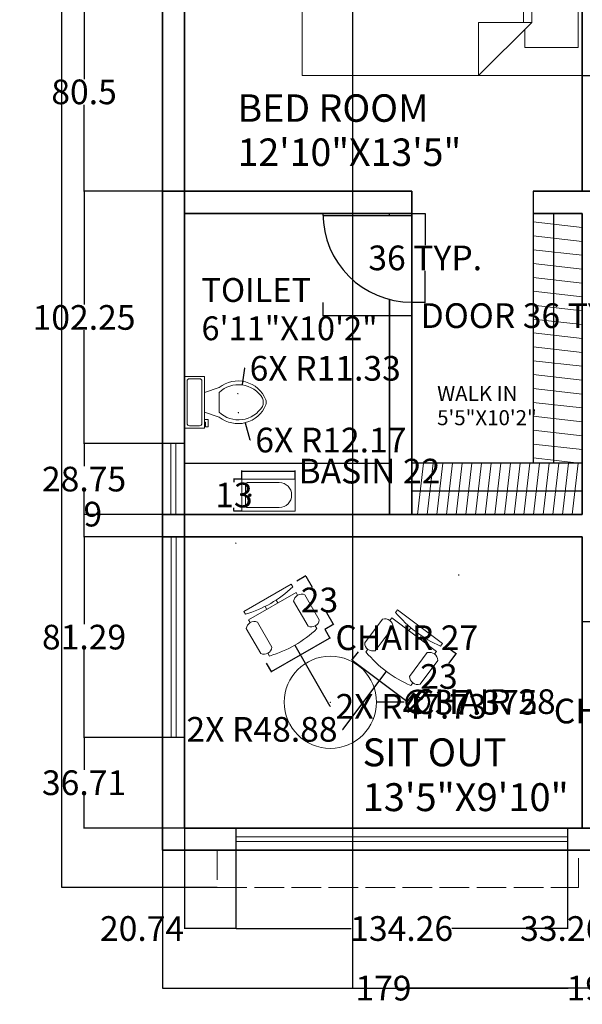
# Model space of a CAD drawing. Units: inches. Extents: x 135 to 880, y 60 to 879.
# Tile 1 of 5: x 135 to 363, y 60 to 459. Entities that reach past the tile are written whole.
import ezdxf

# ---------------------------------------------------------------- set-up
doc = ezdxf.new("R2010")
doc.units = ezdxf.units.IN
doc.header["$MEASUREMENT"] = 0
doc.linetypes.add('ACAD_ISO02W100', pattern=[15, 12, -3])
for name, color, linetype, lineweight in [('A-ANNO-DIMS', 2, 'Continuous', 18), ('A-AREA-IDEN', 7, 'Continuous', 18), ('A-DOOR', 3, 'Continuous', 25), ('A-FLOR-CASE', 32, 'Continuous', 25), ('A-FLOR-CASE-PATT', 252, 'Continuous', 13), ('A-FLOR-FIXT', 9, 'Continuous', 20), ('A-FURN', 8, 'Continuous', 18), ('A-GLAZ', 4, 'Continuous', 18), ('A-ROOF-OVHD', 8, 'ACAD_ISO02W100', 18), ('A-WALL', 7, 'Continuous', 35)]:
    doc.layers.add(name, color=color, linetype=linetype, lineweight=lineweight)
doc.styles.get("Standard").update_dxf_attribs({"font": 'arial.ttf'})
doc.dimstyles.get("Standard").update_dxf_attribs({"dimtxt": 10, "dimasz": 0.18, "dimexe": 0.18, "dimexo": 0.0625, "dimgap": 0.09, "dimtad": 0, "dimtih": 1, "dimtoh": 1, "dimdec": 0, "dimzin": 0, "dimdsep": 46, "dimlunit": 3, "dimtxsty": 'Standard', "dimcen": 0.09, "dimadec": 0, "dimazin": 0, "dimtfac": 1, "dimtdec": 0, "dimtofl": 0, "dimtmove": 0, "dimatfit": 3, "dimfxl": 1, "dimtolj": 1, "dimtzin": 0, "dimarcsym": 0})

# ---------------------------------------------------------------- blocks, each defined once
blk = doc.blocks.new('Chair - Desk')
for p, q in [((-8.5, 0), (-8.5, -1)), ((-8.5, 0), (8.5, 0)), ((8.5, 0), (8.5, -1)), ((-2, -3), (-2, -1.9355)), ((2, -1.9576), (2, -3)), ((-10.5, -5), (-10.5, -14)), ((-8.5, -3), (-8.5, -4)), ((-8.5, -3), (8.5, -3)), ((-6.5, -14), (-6.5, -5)), ((6.5, -5), (6.5, -14)), ((8.5, -3), (8.5, -4)), ((10.5, -14), (10.5, -5)), ((-8.5, -15), (-8.5, -16)), ((8.5, -15), (8.5, -16))]:
    blk.add_line(p, q)
for centre, radius, start, end in [((0, 34.625), 36.625, 256.5803, 283.4197), ((-8.5, -6.5), 2.5, 36.8699, 143.1301), ((8.5, -6.5), 2.5, 36.8699, 143.1301), ((-8.5, -12.5), 2.5, 216.8699, 323.1301), ((8.5, -12.5), 2.5, 216.8699, 323.1301), ((0, 19.625), 36.625, 256.5803, 283.4197)]:
    blk.add_arc(centre, radius, start, end)
blk = doc.blocks.new('Bed - Queen')
for p, q in [((0, -80.00003), (0, 0)), ((0, 0), (59.99999, 0)), ((59.99999, 0), (59.99999, -80.00003)), ((7.99999, -1.2), (28.79998, -1.2)), ((7.99999, -14.4), (7.99999, -1.2)), ((28.79998, -1.2), (28.79998, -14.4)), ((31.19999, -1.2), (51.99999, -1.2)), ((31.19999, -14.4), (31.19999, -1.2)), ((51.99999, -1.2), (51.99999, -16.4)), ((0, -14.4), (44.8, -14.4)), ((44.8, -16.8), (0, -16.8)), ((59.99999, -29.6), (44.8, -14.4)), ((44.8, -14.4), (44.8, -29.6)), ((51.99999, -16.4), (46.79936, -16.4)), ((44.8, -29.6), (59.99999, -29.6)), ((59.99999, -80.00003), (0, -80.00003))]:
    blk.add_line(p, q)
blk = doc.blocks.new('Toilet - top')
for p, q in [((9.5, -6), (9.5, -2)), ((-10, -8.5), (-8, -8.5)), ((-10, -9.5), (-10, -8.5)), ((-7, -9.5), (-10, -9.5)), ((-8, -8.5), (-8, -8)), ((-7, -8), (-7, -9.5)), ((-4, -8), (-6, -14)), ((4, -8), (6, -14)), ((4, -14), (-4, -14))]:
    blk.add_line(p, q)
blk.add_lwpolyline([(10.5, -8), (10.5, 0), (-10.5, 0), (-10.5, -8)], close=True)
for points in [[(-9.5, -2), (-9.5, -6)], [(8.5, -1), (-8.5, -1)], [(-8.5, -7), (8.5, -7)]]:
    blk.add_lwpolyline(points)
for centre, radius, start, end in [((-8.62, -1.88), 0.884, 81.8699, 188.1301), ((8.62, -1.88), 0.884, 351.8699, 98.1301), ((-8.62, -6.12), 0.884, 171.8699, 278.1301), ((8.62, -6.12), 0.884, 261.8699, 8.1301), ((3.52, -21.58), 12.17, 141.4691, 247.9714), ((4.2, -21.82), 11.33, 136.3677, 238.9468), ((-3.52, -21.58), 12.17, 292.0284, 38.5307), ((-4.2, -21.82), 11.33, 301.053, 43.6321), ((0, -27.88), 4, 245.7318, 294.2682), ((0, -29), 4, 254.8605, 285.1395)]:
    blk.add_arc(centre, radius, start, end)
blk = doc.blocks.new('Bath Tub - 26 x 60 in.')
for p, q in [((8, -18), (10, -18)), ((9, -17), (9, -19))]:
    blk.add_line(p, q)
blk.add_lwpolyline([(0, -36), (0, 0), (60, 0), (60, -36)], close=True)
for points in [[(4, -30), (4, -6)], [(6, -4), (42, -4)], [(42, -32), (6, -32)]]:
    blk.add_lwpolyline(points)
for radius in [1.5, 1]:
    blk.add_circle((9, -18), radius)
for centre, radius, start, end in [((5.75, -5.75), 1.77, 81.8699, 188.1301), ((42, -18), 14, 270, 90), ((5.75, -30.25), 1.77, 171.8699, 278.1301)]:
    blk.add_arc(centre, radius, start, end)
blk = doc.blocks.new('DOOR-SWING-36IN')
for p, q in [((36, 36), (0, 36)), ((36, 35), (0, 35))]:
    blk.add_line(p, q)
blk.add_arc((36, 36), 36, 180, 270)
blk = doc.blocks.new('*D8')
at = {"layer": 'A-ANNO-DIMS', "color": 0, "lineweight": -2, "transparency": 16777216}
for p, q in [((258.71, 212.22), (260.83, 208.57)), ((237.19, 195.13), (260.58, 208.63)), ((260.74, 208.72), (260.89, 208.81)), ((260.89, 208.81), (261.07, 208.81)), ((235.02, 198.54), (237.13, 194.89))]:
    blk.add_line(p, q, dxfattribs=at)
at = {"layer": 'A-ANNO-DIMS', "color": 0, "transparency": 16777216}
for points in [[(260.56, 208.66), (260.59, 208.61), (260.74, 208.72)], [(237.18, 195.16), (237.21, 195.11), (237.04, 195.04)]]:
    blk.add_solid(points, dxfattribs=at)
at = {"layer": 'Defpoints', "color": 0, "transparency": 16777216}
for p in [(258.68, 212.28), (260.74, 208.72), (234.98, 198.6)]:
    blk.add_point(p, dxfattribs=at)
at = {"layer": 'A-ANNO-DIMS', "color": 0, "transparency": 16777216, "insert": (291.94, 208.81), "char_height": 10, "attachment_point": 5}
blk.add_mtext('\\A1;CHAIR 27', dxfattribs=at)
blk = doc.blocks.new('*D9')
at = {"layer": 'A-ANNO-DIMS', "color": 0, "lineweight": -2, "transparency": 16777216}
for p, q in [((247.44, 231.87), (251.1, 233.98)), ((251.03, 233.74), (253.59, 229.31)), ((262.15, 214.49), (259.59, 218.91)), ((258.74, 212.31), (262.39, 214.42))]:
    blk.add_line(p, q, dxfattribs=at)
at = {"layer": 'A-ANNO-DIMS', "color": 0, "transparency": 16777216}
for points in [[(251.06, 233.75), (251.01, 233.72), (250.94, 233.89)], [(262.17, 214.5), (262.12, 214.47), (262.24, 214.33)]]:
    blk.add_solid(points, dxfattribs=at)
at = {"layer": 'Defpoints', "color": 0, "transparency": 16777216}
for p in [(247.39, 231.84), (250.94, 233.89), (258.68, 212.28)]:
    blk.add_point(p, dxfattribs=at)
at = {"layer": 'A-ANNO-DIMS', "color": 0, "transparency": 16777216, "insert": (256.59, 224.11), "char_height": 10, "attachment_point": 5}
blk.add_mtext('\\A1;23', dxfattribs=at)
blk = doc.blocks.new('*D10')
at = {"layer": 'A-ANNO-DIMS', "color": 0, "lineweight": -2, "transparency": 16777216}
for p, q in [((272.18, 203.16), (269.58, 199.7)), ((269.83, 199.74), (291.97, 183.14)), ((294.59, 186.34), (292, 182.88)), ((292.11, 183.03), (292.25, 182.92)), ((292.25, 182.92), (292.43, 182.92))]:
    blk.add_line(p, q, dxfattribs=at)
at = {"layer": 'A-ANNO-DIMS', "color": 0, "transparency": 16777216}
for points in [[(269.85, 199.76), (269.82, 199.71), (269.69, 199.84)], [(291.98, 183.16), (291.95, 183.11), (292.11, 183.03)]]:
    blk.add_solid(points, dxfattribs=at)
at = {"layer": 'Defpoints', "color": 0, "transparency": 16777216}
for p in [(272.21, 203.21), (294.63, 186.39), (292.11, 183.03)]:
    blk.add_point(p, dxfattribs=at)
at = {"layer": 'A-ANNO-DIMS', "color": 0, "transparency": 16777216, "insert": (323.31, 182.92), "char_height": 10, "attachment_point": 5}
blk.add_mtext('\\A1;CHAIR 28', dxfattribs=at)
blk = doc.blocks.new('*D11')
at = {"layer": 'A-ANNO-DIMS', "color": 0, "lineweight": -2, "transparency": 16777216}
for p, q in [((308.56, 204.86), (312.02, 202.27)), ((311.77, 202.23), (308.83, 198.32)), ((298.1, 184.01), (301.03, 187.92)), ((294.68, 186.35), (298.14, 183.76))]:
    blk.add_line(p, q, dxfattribs=at)
at = {"layer": 'A-ANNO-DIMS', "color": 0, "transparency": 16777216}
for points in [[(311.74, 202.25), (311.79, 202.21), (311.87, 202.37)], [(298.08, 184.03), (298.13, 184), (297.99, 183.87)]]:
    blk.add_solid(points, dxfattribs=at)
at = {"layer": 'Defpoints', "color": 0, "transparency": 16777216}
for p in [(308.51, 204.9), (311.87, 202.37), (294.63, 186.39)]:
    blk.add_point(p, dxfattribs=at)
at = {"layer": 'A-ANNO-DIMS', "color": 0, "transparency": 16777216, "insert": (304.93, 193.12), "char_height": 10, "attachment_point": 5}
blk.add_mtext('\\A1;23', dxfattribs=at)
blk = doc.blocks.new('*D14')
at = {"layer": 'A-ANNO-DIMS', "color": 0, "lineweight": -2, "transparency": 16777216}
for p, q in [((454.9, 202.13), (411.72, 179.27)), ((458.48, 195.75), (454.97, 202.38)), ((411.4, 179.11), (411.22, 179.11)), ((411.56, 179.19), (411.4, 179.11)), ((414.99, 172.72), (411.48, 179.35))]:
    blk.add_line(p, q, dxfattribs=at)
at = {"layer": 'A-ANNO-DIMS', "color": 0, "transparency": 16777216}
for points in [[(454.88, 202.16), (454.91, 202.11), (455.05, 202.22)], [(411.71, 179.3), (411.73, 179.25), (411.56, 179.19)]]:
    blk.add_solid(points, dxfattribs=at)
at = {"layer": 'Defpoints', "color": 0, "transparency": 16777216}
for p in [(458.51, 195.69), (411.56, 179.19), (415.01, 172.67)]:
    blk.add_point(p, dxfattribs=at)
at = {"layer": 'A-ANNO-DIMS', "color": 0, "transparency": 16777216, "insert": (380.34, 179.11), "char_height": 10, "attachment_point": 5}
blk.add_mtext('\\A1;CHAIR 49', dxfattribs=at)
blk = doc.blocks.new('*D18')
at = {"layer": 'A-ANNO-DIMS', "color": 0, "lineweight": -2, "transparency": 16777216}
for p, q in [((225.19, 273.15), (225.19, 276.5)), ((225.37, 276.32), (246.58, 276.32)), ((246.76, 273.15), (246.76, 276.5)), ((246.76, 276.32), (246.94, 276.32))]:
    blk.add_line(p, q, dxfattribs=at)
at = {"layer": 'A-ANNO-DIMS', "color": 0, "transparency": 16777216}
for points in [[(225.37, 276.35), (225.37, 276.29), (225.19, 276.32)], [(246.58, 276.35), (246.58, 276.29), (246.76, 276.32)]]:
    blk.add_solid(points, dxfattribs=at)
at = {"layer": 'Defpoints', "color": 0, "transparency": 16777216}
for p in [(246.76, 276.32), (225.19, 273.08), (246.76, 273.08)]:
    blk.add_point(p, dxfattribs=at)
at = {"layer": 'A-ANNO-DIMS', "color": 0, "transparency": 16777216, "insert": (276.82, 276.32), "char_height": 10, "attachment_point": 5}
blk.add_mtext('\\A1;BASIN 22', dxfattribs=at)
blk = doc.blocks.new('*D19')
at = {"layer": 'A-ANNO-DIMS', "color": 0, "lineweight": -2, "transparency": 16777216}
for p, q in [((225.13, 273.08), (221.78, 273.08)), ((221.96, 272.9), (221.96, 271.81)), ((225.13, 260.15), (221.78, 260.15)), ((221.96, 260.33), (221.96, 261.42))]:
    blk.add_line(p, q, dxfattribs=at)
at = {"layer": 'A-ANNO-DIMS', "color": 0, "transparency": 16777216}
for points in [[(221.93, 272.9), (221.99, 272.9), (221.96, 273.08)], [(221.93, 260.33), (221.99, 260.33), (221.96, 260.15)]]:
    blk.add_solid(points, dxfattribs=at)
at = {"layer": 'Defpoints', "color": 0, "transparency": 16777216}
for p in [(221.96, 273.08), (225.19, 273.08), (225.19, 260.15)]:
    blk.add_point(p, dxfattribs=at)
at = {"layer": 'A-ANNO-DIMS', "color": 0, "transparency": 16777216, "insert": (221.96, 266.62), "char_height": 10, "attachment_point": 5}
blk.add_mtext('\\A1;13', dxfattribs=at)
blk = doc.blocks.new('*D25')
at = {"layer": 'A-ANNO-DIMS', "color": 0, "lineweight": -2, "transparency": 16777216}
for p, q in [((363.04, 521.66), (380.17, 521.66)), ((379.99, 521.48), (379.99, 484.31)), ((379.99, 436.75), (379.99, 473.92)), ((363.04, 436.57), (380.17, 436.57))]:
    blk.add_line(p, q, dxfattribs=at)
at = {"layer": 'A-ANNO-DIMS', "color": 0, "transparency": 16777216}
for points in [[(379.96, 521.48), (380.02, 521.48), (379.99, 521.66)], [(379.96, 436.75), (380.02, 436.75), (379.99, 436.57)]]:
    blk.add_solid(points, dxfattribs=at)
at = {"layer": 'Defpoints', "color": 0, "transparency": 16777216}
for p in [(362.98, 521.66), (362.98, 436.57), (379.99, 436.57)]:
    blk.add_point(p, dxfattribs=at)
at = {"layer": 'A-ANNO-DIMS', "color": 0, "transparency": 16777216, "insert": (379.99, 479.12), "char_height": 10, "attachment_point": 5}
blk.add_mtext('\\A1;85', dxfattribs=at)
blk = doc.blocks.new('*D32')
at = {"layer": 'A-ANNO-DIMS', "color": 0, "lineweight": -2, "transparency": 16777216}
for p, q in [((257.98, 344.64), (257.98, 339.12)), ((293.98, 344.64), (293.98, 339.12)), ((258.16, 339.3), (293.8, 339.3)), ((293.98, 339.3), (294.16, 339.3))]:
    blk.add_line(p, q, dxfattribs=at)
at = {"layer": 'A-ANNO-DIMS', "color": 0, "transparency": 16777216}
for points in [[(258.16, 339.33), (258.16, 339.27), (257.98, 339.3)], [(293.8, 339.33), (293.8, 339.27), (293.98, 339.3)]]:
    blk.add_solid(points, dxfattribs=at)
at = {"layer": 'Defpoints', "color": 0, "transparency": 16777216}
for p in [(257.98, 344.7), (293.98, 344.7), (293.98, 339.3)]:
    blk.add_point(p, dxfattribs=at)
at = {"layer": 'A-ANNO-DIMS', "color": 0, "transparency": 16777216, "insert": (341.23, 339.3), "char_height": 10, "attachment_point": 5}
blk.add_mtext('\\A1;DOOR 36 TYP.', dxfattribs=at)
blk = doc.blocks.new('*D33')
at = {"layer": 'A-ANNO-DIMS', "color": 0, "lineweight": -2, "transparency": 16777216}
for p, q in [((294.04, 380.7), (299.56, 380.7)), ((299.38, 380.52), (299.38, 367.9)), ((299.38, 344.88), (299.38, 357.5)), ((294.04, 344.7), (299.56, 344.7))]:
    blk.add_line(p, q, dxfattribs=at)
at = {"layer": 'A-ANNO-DIMS', "color": 0, "transparency": 16777216}
for points in [[(299.35, 380.52), (299.41, 380.52), (299.38, 380.7)], [(299.35, 344.88), (299.41, 344.88), (299.38, 344.7)]]:
    blk.add_solid(points, dxfattribs=at)
at = {"layer": 'Defpoints', "color": 0, "transparency": 16777216}
for p in [(293.98, 380.7), (299.38, 380.7), (293.98, 344.7)]:
    blk.add_point(p, dxfattribs=at)
at = {"layer": 'A-ANNO-DIMS', "color": 0, "transparency": 16777216, "insert": (299.38, 362.7), "char_height": 10, "attachment_point": 5}
blk.add_mtext('\\A1;36 TYP.', dxfattribs=at)
blk = doc.blocks.new('*D39')
at = {"layer": 'A-ANNO-DIMS', "color": 0, "lineweight": -2, "transparency": 16777216}
for p, q in [((192.91, 831.7), (152.1, 831.7)), ((152.28, 831.52), (152.28, 474.74)), ((152.28, 107.73), (152.28, 464.52)), ((215.16, 107.55), (152.1, 107.55))]:
    blk.add_line(p, q, dxfattribs=at)
at = {"layer": 'A-ANNO-DIMS', "color": 0, "transparency": 16777216}
for points in [[(152.25, 831.52), (152.31, 831.52), (152.28, 831.7)], [(152.25, 107.73), (152.31, 107.73), (152.28, 107.55)]]:
    blk.add_solid(points, dxfattribs=at)
at = {"layer": 'Defpoints', "color": 0, "transparency": 16777216}
for p in [(152.28, 831.7), (192.98, 831.7), (215.22, 107.55)]:
    blk.add_point(p, dxfattribs=at)
at = {"layer": 'A-ANNO-DIMS', "color": 0, "transparency": 16777216, "insert": (152.28, 469.63), "char_height": 10, "attachment_point": 5}
blk.add_mtext('\\A1;724.1', dxfattribs=at)
blk = doc.blocks.new('*D45')
at = {"layer": 'A-ANNO-DIMS', "color": 0, "lineweight": -2, "transparency": 16777216}
for p, q in [((201.91, 168.41), (161.1, 168.41)), ((161.28, 168.23), (161.28, 155.26)), ((161.28, 131.88), (161.28, 144.86)), ((201.91, 131.7), (161.1, 131.7))]:
    blk.add_line(p, q, dxfattribs=at)
at = {"layer": 'A-ANNO-DIMS', "color": 0, "transparency": 16777216}
for points in [[(161.25, 168.23), (161.31, 168.23), (161.28, 168.41)], [(161.25, 131.88), (161.31, 131.88), (161.28, 131.7)]]:
    blk.add_solid(points, dxfattribs=at)
at = {"layer": 'Defpoints', "color": 0, "transparency": 16777216}
for p in [(161.28, 168.41), (201.98, 168.41), (201.98, 131.7)]:
    blk.add_point(p, dxfattribs=at)
at = {"layer": 'A-ANNO-DIMS', "color": 0, "transparency": 16777216, "insert": (161.28, 150.06), "char_height": 10, "attachment_point": 5}
blk.add_mtext('\\A1;36.71', dxfattribs=at)
blk = doc.blocks.new('*D46')
at = {"layer": 'A-ANNO-DIMS', "color": 0, "lineweight": -2, "transparency": 16777216}
for p, q in [((201.91, 249.7), (161.1, 249.7)), ((161.28, 249.52), (161.28, 214.25)), ((161.28, 168.59), (161.28, 203.86)), ((201.91, 168.41), (161.1, 168.41))]:
    blk.add_line(p, q, dxfattribs=at)
at = {"layer": 'A-ANNO-DIMS', "color": 0, "transparency": 16777216}
for points in [[(161.25, 249.52), (161.31, 249.52), (161.28, 249.7)], [(161.25, 168.59), (161.31, 168.59), (161.28, 168.41)]]:
    blk.add_solid(points, dxfattribs=at)
at = {"layer": 'Defpoints', "color": 0, "transparency": 16777216}
for p in [(161.28, 249.7), (201.98, 249.7), (201.98, 168.41)]:
    blk.add_point(p, dxfattribs=at)
at = {"layer": 'A-ANNO-DIMS', "color": 0, "transparency": 16777216, "insert": (161.28, 209.06), "char_height": 10, "attachment_point": 5}
blk.add_mtext('\\A1;81.29', dxfattribs=at)
blk = doc.blocks.new('*D47')
at = {"layer": 'A-ANNO-DIMS', "color": 0, "lineweight": -2, "transparency": 16777216}
for p, q in [((201.91, 258.7), (161.1, 258.7)), ((161.28, 258.7), (161.28, 258.88)), ((161.28, 258.88), (161.46, 258.88)), ((161.28, 249.88), (161.28, 258.52)), ((201.91, 249.7), (161.1, 249.7))]:
    blk.add_line(p, q, dxfattribs=at)
at = {"layer": 'A-ANNO-DIMS', "color": 0, "transparency": 16777216}
for points in [[(161.25, 258.52), (161.31, 258.52), (161.28, 258.7)], [(161.25, 249.88), (161.31, 249.88), (161.28, 249.7)]]:
    blk.add_solid(points, dxfattribs=at)
at = {"layer": 'Defpoints', "color": 0, "transparency": 16777216}
for p in [(161.28, 258.7), (201.98, 258.7), (201.98, 249.7)]:
    blk.add_point(p, dxfattribs=at)
at = {"layer": 'A-ANNO-DIMS', "color": 0, "transparency": 16777216, "insert": (164.83, 258.88), "char_height": 10, "attachment_point": 5}
blk.add_mtext('\\A1;9', dxfattribs=at)
blk = doc.blocks.new('*D48')
at = {"layer": 'A-ANNO-DIMS', "color": 0, "lineweight": -2, "transparency": 16777216}
for p, q in [((201.91, 287.45), (161.1, 287.45)), ((161.28, 287.27), (161.28, 278.27)), ((161.28, 258.88), (161.28, 267.88)), ((201.91, 258.7), (161.1, 258.7))]:
    blk.add_line(p, q, dxfattribs=at)
at = {"layer": 'A-ANNO-DIMS', "color": 0, "transparency": 16777216}
for points in [[(161.25, 287.27), (161.31, 287.27), (161.28, 287.45)], [(161.25, 258.88), (161.31, 258.88), (161.28, 258.7)]]:
    blk.add_solid(points, dxfattribs=at)
at = {"layer": 'Defpoints', "color": 0, "transparency": 16777216}
for p in [(161.28, 287.45), (201.98, 287.45), (201.98, 258.7)]:
    blk.add_point(p, dxfattribs=at)
at = {"layer": 'A-ANNO-DIMS', "color": 0, "transparency": 16777216, "insert": (161.28, 273.08), "char_height": 10, "attachment_point": 5}
blk.add_mtext('\\A1;28.75', dxfattribs=at)
blk = doc.blocks.new('*D49')
at = {"layer": 'A-ANNO-DIMS', "color": 0, "lineweight": -2, "transparency": 16777216}
for p, q in [((201.91, 389.7), (161.1, 389.7)), ((161.28, 389.52), (161.28, 343.77)), ((161.28, 287.63), (161.28, 333.38)), ((201.91, 287.45), (161.1, 287.45))]:
    blk.add_line(p, q, dxfattribs=at)
at = {"layer": 'A-ANNO-DIMS', "color": 0, "transparency": 16777216}
for points in [[(161.25, 389.52), (161.31, 389.52), (161.28, 389.7)], [(161.25, 287.63), (161.31, 287.63), (161.28, 287.45)]]:
    blk.add_solid(points, dxfattribs=at)
at = {"layer": 'Defpoints', "color": 0, "transparency": 16777216}
for p in [(161.28, 389.7), (201.98, 389.7), (201.98, 287.45)]:
    blk.add_point(p, dxfattribs=at)
at = {"layer": 'A-ANNO-DIMS', "color": 0, "transparency": 16777216, "insert": (161.28, 338.58), "char_height": 10, "attachment_point": 5}
blk.add_mtext('\\A1;102.25', dxfattribs=at)
blk = doc.blocks.new('*D50')
at = {"layer": 'A-ANNO-DIMS', "color": 0, "lineweight": -2, "transparency": 16777216}
for p, q in [((201.91, 470.2), (161.1, 470.2)), ((161.28, 470.02), (161.28, 435.15)), ((161.28, 389.88), (161.28, 424.76)), ((201.91, 389.7), (161.1, 389.7))]:
    blk.add_line(p, q, dxfattribs=at)
at = {"layer": 'A-ANNO-DIMS', "color": 0, "transparency": 16777216}
for points in [[(161.25, 470.02), (161.31, 470.02), (161.28, 470.2)], [(161.25, 389.88), (161.31, 389.88), (161.28, 389.7)]]:
    blk.add_solid(points, dxfattribs=at)
at = {"layer": 'Defpoints', "color": 0, "transparency": 16777216}
for p in [(161.28, 470.2), (201.98, 470.2), (201.98, 389.7)]:
    blk.add_point(p, dxfattribs=at)
at = {"layer": 'A-ANNO-DIMS', "color": 0, "transparency": 16777216, "insert": (161.28, 429.95), "char_height": 10, "attachment_point": 5}
blk.add_mtext('\\A1;80.5', dxfattribs=at)
blk = doc.blocks.new('*D54')
at = {"layer": 'A-ANNO-DIMS', "color": 0, "lineweight": -2, "transparency": 16777216}
for p, q in [((192.98, 122.64), (192.98, 66.67)), ((371.98, 122.64), (371.98, 66.67)), ((193.16, 66.85), (271.8, 66.85)), ((371.8, 66.85), (293.15, 66.85))]:
    blk.add_line(p, q, dxfattribs=at)
at = {"layer": 'A-ANNO-DIMS', "color": 0, "transparency": 16777216}
for points in [[(193.16, 66.88), (193.16, 66.82), (192.98, 66.85)], [(371.8, 66.88), (371.8, 66.82), (371.98, 66.85)]]:
    blk.add_solid(points, dxfattribs=at)
at = {"layer": 'Defpoints', "color": 0, "transparency": 16777216}
for p in [(192.98, 122.7), (371.98, 122.7), (371.98, 66.85)]:
    blk.add_point(p, dxfattribs=at)
at = {"layer": 'A-ANNO-DIMS', "color": 0, "transparency": 16777216, "insert": (282.48, 66.85), "char_height": 10, "attachment_point": 5}
blk.add_mtext('\\A1;179', dxfattribs=at)
blk = doc.blocks.new('*D57')
at = {"layer": 'A-ANNO-DIMS', "color": 0, "lineweight": -2, "transparency": 16777216}
for p, q in [((201.98, 131.64), (201.98, 90.82)), ((222.72, 131.64), (222.72, 90.82)), ((201.98, 91), (201.8, 91)), ((222.54, 91), (202.16, 91))]:
    blk.add_line(p, q, dxfattribs=at)
at = {"layer": 'A-ANNO-DIMS', "color": 0, "transparency": 16777216}
for points in [[(202.16, 91.03), (202.16, 90.97), (201.98, 91)], [(222.54, 91.03), (222.54, 90.97), (222.72, 91)]]:
    blk.add_solid(points, dxfattribs=at)
at = {"layer": 'Defpoints', "color": 0, "transparency": 16777216}
for p in [(201.98, 131.7), (222.72, 131.7), (201.98, 91)]:
    blk.add_point(p, dxfattribs=at)
at = {"layer": 'A-ANNO-DIMS', "color": 0, "transparency": 16777216, "insert": (184.77, 91), "char_height": 10, "attachment_point": 5}
blk.add_mtext('\\A1;20.74', dxfattribs=at)
blk = doc.blocks.new('*D58')
at = {"layer": 'A-ANNO-DIMS', "color": 0, "lineweight": -2, "transparency": 16777216}
for p, q in [((222.72, 131.64), (222.72, 90.82)), ((356.98, 131.64), (356.98, 90.82)), ((222.9, 91), (269.47, 91)), ((356.8, 91), (310.22, 91))]:
    blk.add_line(p, q, dxfattribs=at)
at = {"layer": 'A-ANNO-DIMS', "color": 0, "transparency": 16777216}
for points in [[(222.9, 91.03), (222.9, 90.97), (222.72, 91)], [(356.8, 91.03), (356.8, 90.97), (356.98, 91)]]:
    blk.add_solid(points, dxfattribs=at)
at = {"layer": 'Defpoints', "color": 0, "transparency": 16777216}
for p in [(222.72, 131.7), (356.98, 131.7), (222.72, 91)]:
    blk.add_point(p, dxfattribs=at)
at = {"layer": 'A-ANNO-DIMS', "color": 0, "transparency": 16777216, "insert": (289.85, 91), "char_height": 10, "attachment_point": 5}
blk.add_mtext('\\A1;134.26', dxfattribs=at)
blk = doc.blocks.new('*D59')
at = {"layer": 'A-ANNO-DIMS', "color": 0, "lineweight": -2, "transparency": 16777216}
for p, q in [((371.98, 131.64), (371.98, 90.82)), ((405.23, 131.64), (405.23, 90.82)), ((371.98, 91), (371.8, 91)), ((405.05, 91), (372.16, 91))]:
    blk.add_line(p, q, dxfattribs=at)
at = {"layer": 'A-ANNO-DIMS', "color": 0, "transparency": 16777216}
for points in [[(372.16, 91.03), (372.16, 90.97), (371.98, 91)], [(405.05, 91.03), (405.05, 90.97), (405.23, 91)]]:
    blk.add_solid(points, dxfattribs=at)
at = {"layer": 'Defpoints', "color": 0, "transparency": 16777216}
for p in [(371.98, 131.7), (405.23, 131.7), (371.98, 91)]:
    blk.add_point(p, dxfattribs=at)
at = {"layer": 'A-ANNO-DIMS', "color": 0, "transparency": 16777216, "insert": (354.84, 91), "char_height": 10, "attachment_point": 5}
blk.add_mtext('\\A1;33.26', dxfattribs=at)
blk = doc.blocks.new('*D72')
at = {"layer": 'A-ANNO-DIMS', "color": 0, "lineweight": -2, "transparency": 16777216}
for p, q in [((269.98, 822.64), (269.98, 66.67)), ((465.98, 822.64), (465.98, 66.67)), ((270.16, 66.85), (357.31, 66.85)), ((465.8, 66.85), (378.64, 66.85))]:
    blk.add_line(p, q, dxfattribs=at)
at = {"layer": 'A-ANNO-DIMS', "color": 0, "transparency": 16777216}
for points in [[(270.16, 66.88), (270.16, 66.82), (269.98, 66.85)], [(465.8, 66.88), (465.8, 66.82), (465.98, 66.85)]]:
    blk.add_solid(points, dxfattribs=at)
at = {"layer": 'Defpoints', "color": 0, "transparency": 16777216}
for p in [(269.98, 822.7), (465.98, 822.7), (465.98, 66.85)]:
    blk.add_point(p, dxfattribs=at)
at = {"layer": 'A-ANNO-DIMS', "color": 0, "transparency": 16777216, "insert": (367.98, 66.85), "char_height": 10, "attachment_point": 5}
blk.add_mtext('\\A1;196', dxfattribs=at)
blk = doc.blocks.new('*D78')
at = {"layer": 'A-ANNO-DIMS', "color": 0, "lineweight": -2, "transparency": 16777216}
for p, q in [((260.9, 182.66), (261.08, 182.66)), ((260.99, 182.57), (260.99, 182.75)), ((290.89, 182.66), (279.86, 182.66))]:
    blk.add_line(p, q, dxfattribs=at)
at = {"layer": 'A-ANNO-DIMS', "color": 0, "transparency": 16777216}
blk.add_solid([(279.86, 182.69), (279.86, 182.63), (279.68, 182.66)], dxfattribs=at)
at = {"layer": 'Defpoints', "color": 0, "transparency": 16777216}
for p in [(242.3, 182.66), (279.68, 182.66)]:
    blk.add_point(p, dxfattribs=at)
at = {"layer": 'A-ANNO-DIMS', "color": 0, "transparency": 16777216, "insert": (317.21, 182.66), "char_height": 10, "attachment_point": 5}
blk.add_mtext('\\A1;∅37.375', dxfattribs=at)
blk = doc.blocks.new('*D88')
at = {"layer": 'A-ANNO-DIMS', "color": 0, "lineweight": -2, "transparency": 16777216}
for p, q in [((312.92, 234.26), (313.1, 234.26)), ((313.01, 234.17), (313.01, 234.35)), ((266.09, 171.69), (283.58, 195.01)), ((265.91, 171.69), (266.09, 171.69))]:
    blk.add_line(p, q, dxfattribs=at)
at = {"layer": 'A-ANNO-DIMS', "color": 0, "transparency": 16777216}
blk.add_solid([(283.56, 195.03), (283.61, 194.99), (283.69, 195.16)], dxfattribs=at)
at = {"layer": 'Defpoints', "color": 0, "transparency": 16777216}
for p in [(313.01, 234.26), (283.69, 195.16)]:
    blk.add_point(p, dxfattribs=at)
at = {"layer": 'A-ANNO-DIMS', "color": 0, "transparency": 16777216, "insert": (233.33, 171.69), "char_height": 10, "attachment_point": 5}
blk.add_mtext('\\A1;2X R48.88', dxfattribs=at)
blk = doc.blocks.new('*D89')
at = {"layer": 'A-ANNO-DIMS', "color": 0, "lineweight": -2, "transparency": 16777216}
for p, q in [((222.66, 247.15), (222.84, 247.15)), ((222.75, 247.06), (222.75, 247.24)), ((260.93, 181.01), (246.71, 205.66)), ((261.11, 181.01), (260.93, 181.01))]:
    blk.add_line(p, q, dxfattribs=at)
at = {"layer": 'A-ANNO-DIMS', "color": 0, "transparency": 16777216}
blk.add_solid([(246.73, 205.67), (246.68, 205.64), (246.62, 205.81)], dxfattribs=at)
at = {"layer": 'Defpoints', "color": 0, "transparency": 16777216}
for p in [(222.75, 247.15), (246.62, 205.81)]:
    blk.add_point(p, dxfattribs=at)
at = {"layer": 'A-ANNO-DIMS', "color": 0, "transparency": 16777216, "insert": (293.69, 181.01), "char_height": 10, "attachment_point": 5}
blk.add_mtext('\\A1;2X R47.73', dxfattribs=at)
blk = doc.blocks.new('*D90')
at = {"layer": 'A-ANNO-DIMS', "color": 0, "lineweight": -2, "transparency": 16777216}
for p, q in [((223.47, 307.72), (223.65, 307.72)), ((223.56, 307.63), (223.56, 307.81)), ((228.5, 288.89), (226.69, 295.78)), ((228.68, 288.89), (228.5, 288.89))]:
    blk.add_line(p, q, dxfattribs=at)
at = {"layer": 'A-ANNO-DIMS', "color": 0, "transparency": 16777216}
blk.add_solid([(226.72, 295.78), (226.66, 295.77), (226.65, 295.95)], dxfattribs=at)
at = {"layer": 'Defpoints', "color": 0, "transparency": 16777216}
for p in [(223.56, 307.72), (226.65, 295.95)]:
    blk.add_point(p, dxfattribs=at)
at = {"layer": 'A-ANNO-DIMS', "color": 0, "transparency": 16777216, "insert": (261.2, 288.89), "char_height": 10, "attachment_point": 5}
blk.add_mtext('\\A1;6X R12.17', dxfattribs=at)
blk = doc.blocks.new('*D91')
at = {"layer": 'A-ANNO-DIMS', "color": 0, "lineweight": -2, "transparency": 16777216}
for p, q in [((226.21, 317.96), (225.33, 311.41)), ((226.39, 317.96), (226.21, 317.96)), ((223.7, 300), (223.88, 300)), ((223.79, 299.91), (223.79, 300.09))]:
    blk.add_line(p, q, dxfattribs=at)
at = {"layer": 'A-ANNO-DIMS', "color": 0, "transparency": 16777216}
blk.add_solid([(225.3, 311.41), (225.36, 311.4), (225.3, 311.23)], dxfattribs=at)
at = {"layer": 'Defpoints', "color": 0, "transparency": 16777216}
for p in [(225.3, 311.23), (223.79, 300)]:
    blk.add_point(p, dxfattribs=at)
at = {"layer": 'A-ANNO-DIMS', "color": 0, "transparency": 16777216, "insert": (258.91, 317.96), "char_height": 10, "attachment_point": 5}
blk.add_mtext('\\A1;6X R11.33', dxfattribs=at)

msp = doc.modelspace()

# ---------------------------------------------------------------- hatches: boundary and pattern name
at = {"layer": 'A-FLOR-CASE-PATT'}
h = msp.add_hatch(dxfattribs=at)
h.set_pattern_fill('ANSI31', color=256, scale=44.7024, angle=128.535, style=0)
h.paths.add_polyline_path([(343.1077, 279.554), (362.9753, 279.554), (362.9753, 377.5427), (343.1077, 379.794)])
h = msp.add_hatch(dxfattribs=at)
h.set_pattern_fill('ANSI31', color=256, scale=31.0859, angle=38.3327, style=0)
h.paths.add_polyline_path([(294.5097, 258.7014), (360.6258, 258.7014), (362.9753, 278.8009), (362.9753, 279.554), (296.9472, 279.554)])

# ---------------------------------------------------------------- linework, layer by layer
at = {"layer": 'A-DOOR'}
for p, q in [((284.9753, 379.7014), (284.9753, 380.7014)), ((362.9753, 215.4206), (371.9753, 215.4206))]:
    msp.add_line(p, q, dxfattribs=at)
at = {"layer": 'A-FLOR-CASE'}
for p, q in [((343.1077, 389.7014), (343.1077, 279.554)), ((351.3602, 380.7014), (351.3602, 279.554)), ((201.9753, 279.554), (284.9753, 279.554)), ((362.9753, 279.554), (293.9753, 279.554)), ((293.9753, 268.3657), (362.9753, 268.3657))]:
    msp.add_line(p, q, dxfattribs=at)
at = {"layer": 'A-FURN'}
msp.add_circle((260.9901, 182.6632), 18.6875, dxfattribs=at)
at = {"layer": 'A-GLAZ'}
for p, q in [((192.9753, 287.4498), (201.9753, 287.4498)), ((196.4753, 287.4498), (196.4753, 258.7014)), ((198.4753, 287.4498), (198.4753, 258.7014)), ((196.5902, 249.7014), (196.5902, 168.4132)), ((198.5902, 249.7014), (198.5902, 168.4132)), ((201.9753, 168.4132), (192.9753, 168.4132)), ((222.715, 131.7014), (222.715, 122.7014)), ((356.9766, 131.7014), (356.9766, 122.7014)), ((222.715, 128.2014), (356.9766, 128.2014)), ((222.715, 126.2014), (356.9766, 126.2014))]:
    msp.add_line(p, q, dxfattribs=at)
at = {"layer": 'A-ROOF-OVHD'}
for p, q in [((215.2242, 122.7014), (215.2242, 107.553)), ((361.4436, 107.553), (361.4436, 122.7014)), ((215.2242, 107.553), (361.4436, 107.553))]:
    msp.add_line(p, q, dxfattribs=at)
at = {"layer": 'A-WALL'}
for p, q in [((192.9753, 389.7014), (192.9753, 559.7014)), ((201.9753, 389.7014), (201.9753, 550.7014)), ((362.9753, 550.7014), (362.9753, 389.7014)), ((192.9753, 258.7014), (192.9753, 389.7014)), ((293.9753, 389.7014), (192.9753, 389.7014)), ((201.9753, 380.7014), (201.9753, 389.7014)), ((293.9753, 258.7014), (293.9753, 389.7014)), ((371.9753, 389.7014), (343.1077, 389.7014)), ((201.9753, 258.7014), (201.9753, 380.7014)), ((293.9753, 380.7014), (201.9753, 380.7014)), ((362.9753, 380.7014), (343.1077, 380.7014)), ((362.9753, 258.7014), (362.9753, 380.7014)), ((284.9753, 258.7014), (284.9753, 345.8445)), ((362.9753, 258.7014), (192.9753, 258.7014)), ((192.9753, 258.7014), (192.9753, 122.7014)), ((201.9753, 249.7014), (201.9753, 258.7014)), ((201.9753, 258.7014), (284.9753, 258.7014)), ((201.9753, 258.7014), (284.9753, 258.7014)), ((293.9753, 258.7014), (358.9753, 258.7014)), ((362.9753, 249.7014), (192.9753, 249.7014)), ((201.9753, 249.7014), (201.9753, 131.7014)), ((362.9753, 131.7014), (362.9753, 249.7014)), ((201.9753, 131.7014), (362.9753, 131.7014)), ((362.9753, 131.7014), (371.9753, 131.7014)), ((192.9753, 122.7014), (371.9753, 122.7014))]:
    msp.add_line(p, q, dxfattribs=at)

# ---------------------------------------------------------------- block references
at = {"layer": 'A-DOOR'}
msp.add_blockref('DOOR-SWING-36IN', (257.975, 344.701), dxfattribs=at)
at = {"layer": 'A-FLOR-FIXT', "rotation": 90}
msp.add_blockref('Toilet - top', (201.9753, 304.1995), dxfattribs=at)
at = {"layer": 'A-FLOR-FIXT', "xscale": 0.3593938895154072, "yscale": 0.3593938895154072, "zscale": 0.3593938895154072}
msp.add_blockref('Bath Tub - 26 x 60 in.', (225.1938, 273.0849), dxfattribs=at)
at = {"layer": 'A-FURN'}
for name, p, xscale, yscale, zscale, rotation in [('Bed - Queen', (362.9753, 521.6594), 1.418135637024811, 1.418135637024811, 1.418135637024811, 270), ('Chair - Desk', (235.5402, 224.9984), 1.303079767215541, 1.303079767215541, 1.303079767215541, 29.99999999999987), ('Chair - Desk', (297.301, 213.304), 1.334490941934616, 1.334490941934616, 1.334490941934616, 323.1301023541558)]:
    msp.add_blockref(name, p, dxfattribs=dict(at, xscale=xscale, yscale=yscale, zscale=zscale, rotation=rotation))

# ---------------------------------------------------------------- texts
at = {"layer": 'A-AREA-IDEN'}
for s, height, p in [('BED ROOM ', 11.13459, (223.4246, 417.8258)), ('12\'10"X13\'5"', 11.134589, (223.4246, 399.9391)), ('TOILET ', 9.66409, (208.8186, 344.8533)), ('6\'11"X10\'2"', 9.664086, (208.8186, 329.3288)), ('WALK IN ', 6.08951, (304.223, 304.6932)), ('5\'5"X10\'2"', 6.08951, (304.223, 294.9109)), ('SIT OUT ', 11.31212, (274.0248, 156.729)), ('13\'5"X9\'10"', 11.312115, (274.0248, 138.557))]:
    msp.add_text(s, height=height, dxfattribs=at).set_placement(p)

# ---------------------------------------------------------------- dimensions: what is measured, and where the dimension line sits
at = {"layer": 'A-ANNO-DIMS'}
for base, p1, p2, angle, override, picture, middle in [((152.2753, 831.7014), (215.2242, 107.553), (192.9753, 831.7014), 90, {"dimdec": 1, "dimlfac": 1, "dimrnd": 0, "dimzin": 0, "dimdsep": 46, "dimlunit": 2}, '*D39', (152.2753, 469.6272)), ((379.993, 436.5713), (362.9753, 521.6594), (362.9753, 436.5713), 270, {"dimdec": 0, "dimlfac": 1, "dimrnd": 0, "dimzin": 0, "dimdsep": 46, "dimlunit": 2}, '*D25', (379.993, 479.1154)), ((161.2753, 470.2014), (201.9753, 389.7014), (201.9753, 470.2014), 90, {"dimdec": 1, "dimlfac": 1, "dimrnd": 0, "dimzin": 0, "dimdsep": 46, "dimlunit": 2}, '*D50', (161.2753, 429.9514)), ((161.2753, 389.7014), (201.9753, 287.4498), (201.9753, 389.7014), 90, {"dimdec": 2, "dimlfac": 1, "dimrnd": 0, "dimzin": 0, "dimdsep": 46, "dimlunit": 2}, '*D49', (161.2753, 338.5756)), ((161.2753, 287.4498), (201.9753, 258.7014), (201.9753, 287.4498), 90, {"dimdec": 2, "dimlfac": 1, "dimrnd": 0, "dimzin": 0, "dimdsep": 46, "dimlunit": 2}, '*D48', (161.2753, 273.0756)), ((221.9592, 273.0849), (225.1938, 260.1468), (225.1938, 273.0849), 90, {"dimdec": 0, "dimlfac": 1, "dimrnd": 0, "dimzin": 0, "dimdsep": 46, "dimlunit": 2}, '*D19', (221.9592, 266.6158)), ((161.2753, 258.7014), (201.9753, 249.7014), (201.9753, 258.7014), 90, {"dimdec": 0, "dimlfac": 1, "dimrnd": 0, "dimzin": 0, "dimdsep": 46, "dimlunit": 2}, '*D47', (164.8332, 258.8814)), ((161.2753, 249.7014), (201.9753, 168.4132), (201.9753, 249.7014), 90, {"dimdec": 2, "dimlfac": 1, "dimrnd": 0, "dimzin": 0, "dimdsep": 46, "dimlunit": 2}, '*D46', (161.2753, 209.0573)), ((250.9443, 233.892), (258.6828, 212.2789), (247.3895, 231.8396), 120, {"dimdec": 0, "dimlfac": 1, "dimrnd": 0, "dimzin": 0, "dimdsep": 46, "dimlunit": 2}, '*D9', (256.5909, 224.1116)), ((311.8737, 202.3745), (294.632, 186.3918), (308.5107, 204.8967), 53.130102, {"dimdec": 0, "dimlfac": 1, "dimrnd": 0, "dimzin": 0, "dimdsep": 46, "dimlunit": 2}, '*D11', (304.9343, 193.1221)), ((161.2753, 168.4132), (201.9753, 131.7014), (201.9753, 168.4132), 90, {"dimdec": 2, "dimlfac": 1, "dimrnd": 0, "dimzin": 0, "dimdsep": 46, "dimlunit": 2}, '*D45', (161.2753, 150.0573)), ((201.9753, 91.0014), (222.715, 131.7014), (201.9753, 131.7014), 180, {"dimdec": 2, "dimlfac": 1, "dimrnd": 0, "dimzin": 0, "dimdsep": 46, "dimlunit": 2}, '*D57', (184.7681, 91.0014)), ((222.715, 91.0014), (356.9766, 131.7014), (222.715, 131.7014), 180, {"dimdec": 2, "dimlfac": 1, "dimrnd": 0, "dimzin": 0, "dimdsep": 46, "dimlunit": 2}, '*D58', (289.8458, 91.0014)), ((371.9753, 91.0014), (405.2334, 131.7014), (371.9753, 131.7014), 180, {"dimdec": 2, "dimlfac": 1, "dimrnd": 0, "dimzin": 0, "dimdsep": 46, "dimlunit": 2}, '*D59', (354.8397, 91.0014))]:
    dim = msp.add_linear_dim(base=base, p1=p1, p2=p2, angle=angle, dimstyle='Standard', override=override, dxfattribs=at)
    dim.commit()
    dim.dimension.update_dxf_attribs({"geometry": picture, "text_midpoint": middle})
for base, p1, p2, picture, middle in [((465.9753, 66.853), (269.9753, 822.7014), (465.9753, 822.7014), '*D72', (367.9753, 66.853)), ((371.9753, 66.853), (192.9753, 122.7014), (371.9753, 122.7014), '*D54', (282.4753, 66.853))]:
    dim = msp.add_linear_dim(base=base, p1=p1, p2=p2, dimstyle='Standard', override={"dimdec": 0, "dimlfac": 1, "dimrnd": 0, "dimzin": 0, "dimdsep": 46, "dimlunit": 2}, dxfattribs=at)
    dim.commit()
    dim.dimension.update_dxf_attribs({"geometry": picture, "text_midpoint": middle})
for base, p1, p2, angle, text, picture, middle in [((299.3753, 380.7014), (293.9753, 344.7014), (293.9753, 380.7014), 90, '<> TYP.', '*D33', (299.3753, 362.7014)), ((260.7352, 208.7242), (234.9843, 198.5966), (258.6828, 212.2789), 30, 'CHAIR <>', '*D8', (291.9387, 208.8142)), ((292.1098, 183.0289), (272.2126, 203.2064), (294.632, 186.3918), 323.130102, 'CHAIR <>', '*D10', (323.3117, 182.9209)), ((411.5603, 179.1894), (458.5089, 195.6918), (415.0143, 172.6652), 207.897271, 'CHAIR <>', '*D14', (380.3433, 179.1052))]:
    dim = msp.add_linear_dim(base=base, p1=p1, p2=p2, angle=angle, text=text, dimstyle='Standard', override={"dimdec": 0, "dimlfac": 1, "dimrnd": 0, "dimzin": 0, "dimdsep": 46, "dimlunit": 2}, dxfattribs=at)
    dim.commit()
    dim.dimension.update_dxf_attribs({"geometry": picture, "text_midpoint": middle})
for base, p1, p2, text, picture, middle in [((293.9753, 339.3014), (257.9753, 344.7014), (293.9753, 344.7014), 'DOOR <> TYP.', '*D32', (341.2303, 339.3014)), ((246.7574, 276.3195), (225.1938, 273.0849), (246.7574, 273.0849), 'BASIN <>', '*D18', (276.8194, 276.3195))]:
    dim = msp.add_linear_dim(base=base, p1=p1, p2=p2, text=text, dimstyle='Standard', override={"dimdec": 0, "dimlfac": 1, "dimrnd": 0, "dimzin": 0, "dimdsep": 46, "dimlunit": 2}, dxfattribs=at)
    dim.commit()
    dim.dimension.update_dxf_attribs({"geometry": picture, "text_midpoint": middle})
for center, mpoint, text, picture, middle in [((223.7927, 299.9996), (225.302, 311.2278), '6X <>', '*D91', (258.9059, 317.9647)), ((223.5558, 307.719), (226.6479, 295.9494), '6X <>', '*D90', (261.2015, 288.8876)), ((222.7538, 247.1452), (246.6161, 205.8138), '2X <>', '*D89', (293.6899, 181.0149)), ((313.0146, 234.2555), (283.689, 195.1551), '2X <>', '*D88', (233.3271, 171.6948))]:
    dim = msp.add_radius_dim(center=center, mpoint=mpoint, text=text, dimstyle='Standard', override={"dimdec": 2, "dimlfac": 1, "dimrnd": 0, "dimzin": 0, "dimdsep": 46, "dimlunit": 2}, dxfattribs=at)
    dim.commit()
    dim.dimension.update_dxf_attribs({"geometry": picture, "text_midpoint": middle, "dimtype": 164})
dim = msp.add_diameter_dim_2p(p1=(242.3026, 182.6633), p2=(279.6777, 182.663), dimstyle='Standard', override={"dimdec": 3, "dimlfac": 1, "dimrnd": 0, "dimzin": 0, "dimdsep": 46, "dimlunit": 2}, dxfattribs=at)
dim.commit()
dim.dimension.update_dxf_attribs({"geometry": '*D78', "text_midpoint": (290.8902, 182.6629), "dimtype": 163})

doc.saveas('drawing.dxf')
